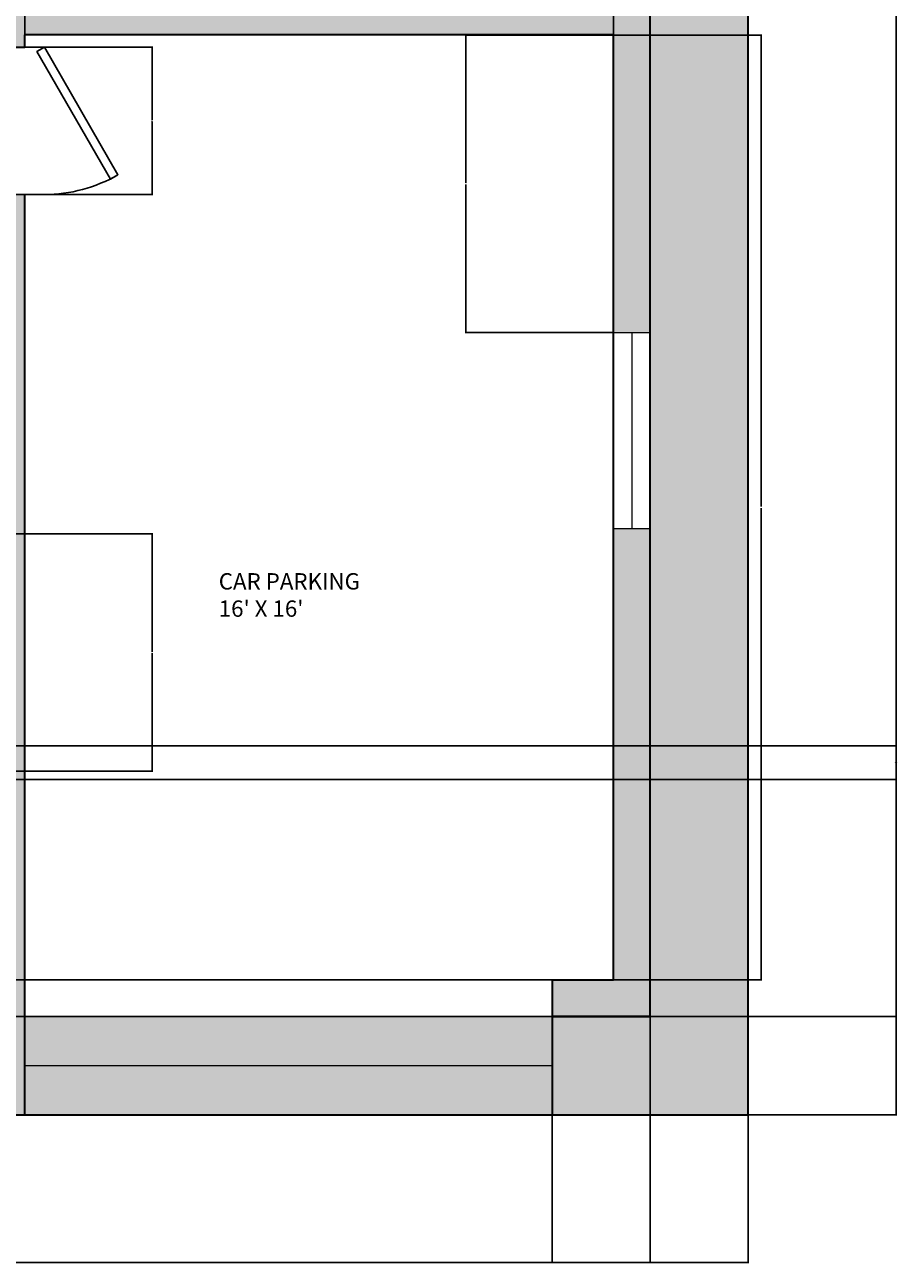
# Model space of a CAD drawing. Units: inches. Extents: x -7 to 546, y -27 to 766.
# Tile 4 of 9: x 332 to 546, y -27 to 276. Entities that reach past the tile are written whole.
import ezdxf

# ---------------------------------------------------------------- set-up
doc = ezdxf.new("R2010")
doc.units = ezdxf.units.IN
doc.header["$MEASUREMENT"] = 0
for name, color, linetype, lineweight in [('A-ANNO-DIMS', 2, 'Continuous', 18), ('A-AREA-IDEN', 7, 'Continuous', 18), ('A-WALL', 7, 'Continuous', 35), ('C-PROP', 7, 'Continuous', 35), ('doors', 40, 'Continuous', 25), ('L-PAVE', 7, 'Continuous', 18), ('window', 30, 'Continuous', 20)]:
    doc.layers.add(name, color=color, linetype=linetype, lineweight=lineweight)
for name, color, linetype, lineweight, true_color in [('A-FLOR-PATT', 143, 'Continuous', 13, 0x7aafdf), ('A-WALL-PATT', 251, 'Continuous', 13, 0x636466), ('L-PLNT-PATT', 85, 'Continuous', 13, 0x58ba48)]:
    doc.layers.add(name, color=color, linetype=linetype, lineweight=lineweight, true_color=true_color)
doc.styles.get("Standard").update_dxf_attribs({"font": 'arial.ttf'})
doc.dimstyles.get("Standard").update_dxf_attribs({"dimtxt": 0.18, "dimasz": 0.18, "dimexe": 0.18, "dimexo": 0.0625, "dimgap": 0.09, "dimtad": 0, "dimtih": 1, "dimtoh": 1, "dimdec": 4, "dimzin": 0, "dimdsep": 46, "dimtxsty": 'Standard', "dimcen": 0.09, "dimadec": 0, "dimazin": 0, "dimtfac": 1, "dimtdec": 4, "dimtofl": 0, "dimtmove": 0, "dimatfit": 3, "dimfxl": 1, "dimtolj": 1, "dimtzin": 0, "dimarcsym": 0})

# ---------------------------------------------------------------- blocks, each defined once
blk = doc.blocks.new('*U10')
for p, q in [((0, 0), (0, -100)), ((750, 0), (750, -100))]:
    blk.add_line(p, q)
blk.add_lwpolyline([(0, 0), (649.5, 375), (671.4, 337.1), (21.9, -37.9)], close=True)
blk.add_arc((0, 0), 750, 0, 30)
blk = doc.blocks.new('WIN-48IN')
for p, q in [((0, 9), (0, 0)), ((48, 9), (0, 9)), ((0, 9), (0, 4.5)), ((48, 0), (48, 9)), ((0, 4.5), (48, 4.5)), ((0, 0), (48, 0))]:
    blk.add_line(p, q)
blk = doc.blocks.new('*D30')
at = {"layer": 'A-ANNO-DIMS', "color": 0, "lineweight": -2, "transparency": 16777216}
for p, q in [((29.23, 9.68), (29.23, -26.56)), ((509.23, 9.68), (509.23, -26.56)), ((29.41, -26.38), (268.94, -26.38)), ((509.05, -26.38), (269.52, -26.38))]:
    blk.add_line(p, q, dxfattribs=at)
at = {"layer": 'A-ANNO-DIMS', "color": 0, "transparency": 16777216}
for points in [[(29.41, -26.35), (29.41, -26.41), (29.23, -26.38)], [(509.05, -26.35), (509.05, -26.41), (509.23, -26.38)]]:
    blk.add_solid(points, dxfattribs=at)
at = {"layer": 'Defpoints', "color": 0, "transparency": 16777216}
for p in [(29.23, 9.74), (509.23, 9.74), (509.23, -26.38)]:
    blk.add_point(p, dxfattribs=at)
at = {"layer": 'A-ANNO-DIMS', "color": 0, "transparency": 16777216, "insert": (269.23, -26.38), "char_height": 0.18, "attachment_point": 5}
blk.add_mtext('\\A1;480', dxfattribs=at)
blk = doc.blocks.new('*D33')
at = {"layer": 'A-ANNO-DIMS', "color": 0, "lineweight": -2, "transparency": 16777216}
for p, q in [((485.29, 705.74), (545.54, 705.74)), ((545.36, 705.56), (545.36, 357.93)), ((545.36, 9.92), (545.36, 357.56)), ((461.29, 9.74), (545.54, 9.74))]:
    blk.add_line(p, q, dxfattribs=at)
at = {"layer": 'A-ANNO-DIMS', "color": 0, "transparency": 16777216}
for points in [[(545.33, 705.56), (545.39, 705.56), (545.36, 705.74)], [(545.33, 9.92), (545.39, 9.92), (545.36, 9.74)]]:
    blk.add_solid(points, dxfattribs=at)
at = {"layer": 'Defpoints', "color": 0, "transparency": 16777216}
for p in [(485.23, 705.74), (461.23, 9.74), (545.36, 9.74)]:
    blk.add_point(p, dxfattribs=at)
at = {"layer": 'A-ANNO-DIMS', "color": 0, "transparency": 16777216, "insert": (545.36, 357.74), "char_height": 0.18, "attachment_point": 5}
blk.add_mtext('\\A1;696', dxfattribs=at)
blk = doc.blocks.new('*D57')
at = {"layer": 'A-ANNO-DIMS', "color": 0, "lineweight": -2, "transparency": 16777216}
for p, q in [((332.23, 273.81), (332.23, 766.05)), ((332.41, 765.87), (403.95, 765.87)), ((476.05, 765.87), (404.51, 765.87)), ((476.23, 273.81), (476.23, 766.05))]:
    blk.add_line(p, q, dxfattribs=at)
at = {"layer": 'A-ANNO-DIMS', "color": 0, "transparency": 16777216}
for points in [[(332.41, 765.9), (332.41, 765.84), (332.23, 765.87)], [(476.05, 765.9), (476.05, 765.84), (476.23, 765.87)]]:
    blk.add_solid(points, dxfattribs=at)
at = {"layer": 'Defpoints', "color": 0, "transparency": 16777216}
for p in [(476.23, 765.87), (332.23, 273.74), (476.23, 273.74)]:
    blk.add_point(p, dxfattribs=at)
at = {"layer": 'A-ANNO-DIMS', "color": 0, "transparency": 16777216, "insert": (404.23, 765.87), "char_height": 0.18, "attachment_point": 5}
blk.add_mtext('\\A1;144', dxfattribs=at)
blk = doc.blocks.new('*D58')
at = {"layer": 'A-ANNO-DIMS', "color": 0, "lineweight": -2, "transparency": 16777216}
for p, q in [((476.29, 273.74), (512.54, 273.74)), ((512.36, 273.56), (512.36, 158.43)), ((512.36, 42.92), (512.36, 158.06)), ((476.29, 42.74), (512.54, 42.74))]:
    blk.add_line(p, q, dxfattribs=at)
at = {"layer": 'A-ANNO-DIMS', "color": 0, "transparency": 16777216}
for points in [[(512.33, 273.56), (512.39, 273.56), (512.36, 273.74)], [(512.33, 42.92), (512.39, 42.92), (512.36, 42.74)]]:
    blk.add_solid(points, dxfattribs=at)
at = {"layer": 'Defpoints', "color": 0, "transparency": 16777216}
for p in [(476.23, 273.74), (476.23, 42.74), (512.36, 42.74)]:
    blk.add_point(p, dxfattribs=at)
at = {"layer": 'A-ANNO-DIMS', "color": 0, "transparency": 16777216, "insert": (512.36, 158.24), "char_height": 0.18, "attachment_point": 5}
blk.add_mtext('\\A1;231', dxfattribs=at)
blk = doc.blocks.new('*D59')
at = {"layer": 'A-ANNO-DIMS', "color": 0, "lineweight": -2, "transparency": 16777216}
for p, q in [((327.29, 151.74), (363.54, 151.74)), ((363.36, 151.56), (363.36, 122.93)), ((363.36, 93.92), (363.36, 122.56)), ((327.29, 93.74), (363.54, 93.74))]:
    blk.add_line(p, q, dxfattribs=at)
at = {"layer": 'A-ANNO-DIMS', "color": 0, "transparency": 16777216}
for points in [[(363.33, 151.56), (363.39, 151.56), (363.36, 151.74)], [(363.33, 93.92), (363.39, 93.92), (363.36, 93.74)]]:
    blk.add_solid(points, dxfattribs=at)
at = {"layer": 'Defpoints', "color": 0, "transparency": 16777216}
for p in [(327.23, 151.74), (327.23, 93.74), (363.36, 93.74)]:
    blk.add_point(p, dxfattribs=at)
at = {"layer": 'A-ANNO-DIMS', "color": 0, "transparency": 16777216, "insert": (363.36, 122.74), "char_height": 0.18, "attachment_point": 5}
blk.add_mtext('\\A1;58', dxfattribs=at)
blk = doc.blocks.new('*D60')
at = {"layer": 'A-ANNO-DIMS', "color": 0, "lineweight": -2, "transparency": 16777216}
for p, q in [((327.29, 270.74), (363.54, 270.74)), ((363.36, 270.56), (363.36, 252.93)), ((363.36, 234.92), (363.36, 252.56)), ((327.29, 234.74), (363.54, 234.74))]:
    blk.add_line(p, q, dxfattribs=at)
at = {"layer": 'A-ANNO-DIMS', "color": 0, "transparency": 16777216}
for points in [[(363.33, 270.56), (363.39, 270.56), (363.36, 270.74)], [(363.33, 234.92), (363.39, 234.92), (363.36, 234.74)]]:
    blk.add_solid(points, dxfattribs=at)
at = {"layer": 'Defpoints', "color": 0, "transparency": 16777216}
for p in [(327.23, 270.74), (327.23, 234.74), (363.36, 234.74)]:
    blk.add_point(p, dxfattribs=at)
at = {"layer": 'A-ANNO-DIMS', "color": 0, "transparency": 16777216, "insert": (363.36, 252.74), "char_height": 0.18, "attachment_point": 5}
blk.add_mtext('\\A1;36', dxfattribs=at)
blk = doc.blocks.new('*D63')
at = {"layer": 'A-ANNO-DIMS', "color": 0, "lineweight": -2, "transparency": 16777216}
for p, q in [((476.17, 273.74), (439.93, 273.74)), ((440.11, 273.56), (440.11, 237.57)), ((440.11, 201.21), (440.11, 237.21)), ((476.17, 201.03), (439.93, 201.03))]:
    blk.add_line(p, q, dxfattribs=at)
at = {"layer": 'A-ANNO-DIMS', "color": 0, "transparency": 16777216}
for points in [[(440.08, 273.56), (440.14, 273.56), (440.11, 273.74)], [(440.08, 201.21), (440.14, 201.21), (440.11, 201.03)]]:
    blk.add_solid(points, dxfattribs=at)
at = {"layer": 'Defpoints', "color": 0, "transparency": 16777216}
for p in [(440.11, 273.74), (476.23, 273.74), (476.23, 201.03)]:
    blk.add_point(p, dxfattribs=at)
at = {"layer": 'A-ANNO-DIMS', "color": 0, "transparency": 16777216, "insert": (440.11, 237.39), "char_height": 0.18, "attachment_point": 5}
blk.add_mtext('\\A1;72.71', dxfattribs=at)
blk = doc.blocks.new('*D64')
at = {"layer": 'A-ANNO-DIMS', "color": 0, "lineweight": -2, "transparency": 16777216}
for p, q in [((461.23, 33.68), (461.23, -26.56)), ((485.23, 33.68), (485.23, -26.56)), ((461.41, -26.38), (473.01, -26.38)), ((485.05, -26.38), (473.45, -26.38))]:
    blk.add_line(p, q, dxfattribs=at)
at = {"layer": 'A-ANNO-DIMS', "color": 0, "transparency": 16777216}
for points in [[(461.41, -26.35), (461.41, -26.41), (461.23, -26.38)], [(485.05, -26.35), (485.05, -26.41), (485.23, -26.38)]]:
    blk.add_solid(points, dxfattribs=at)
at = {"layer": 'Defpoints', "color": 0, "transparency": 16777216}
for p in [(461.23, 33.74), (485.23, 33.74), (461.23, -26.38)]:
    blk.add_point(p, dxfattribs=at)
at = {"layer": 'A-ANNO-DIMS', "color": 0, "transparency": 16777216, "insert": (473.23, -26.38), "char_height": 0.18, "attachment_point": 5}
blk.add_mtext('\\A1;24', dxfattribs=at)
blk = doc.blocks.new('*D65')
at = {"layer": 'A-ANNO-DIMS', "color": 0, "lineweight": -2, "transparency": 16777216}
for p, q in [((461.17, 42.74), (-7.07, 42.74)), ((-6.89, 42.56), (-6.89, 38.43)), ((-6.89, 33.92), (-6.89, 38.06)), ((461.17, 33.74), (-7.07, 33.74))]:
    blk.add_line(p, q, dxfattribs=at)
at = {"layer": 'A-ANNO-DIMS', "color": 0, "transparency": 16777216}
for points in [[(-6.92, 42.56), (-6.86, 42.56), (-6.89, 42.74)], [(-6.92, 33.92), (-6.86, 33.92), (-6.89, 33.74)]]:
    blk.add_solid(points, dxfattribs=at)
at = {"layer": 'Defpoints', "color": 0, "transparency": 16777216}
for p in [(-6.89, 42.74), (461.23, 42.74), (461.23, 33.74)]:
    blk.add_point(p, dxfattribs=at)
at = {"layer": 'A-ANNO-DIMS', "color": 0, "transparency": 16777216, "insert": (-6.89, 38.24), "char_height": 0.18, "attachment_point": 5}
blk.add_mtext('\\A1;9', dxfattribs=at)
blk = doc.blocks.new('*D82')
at = {"layer": 'A-ANNO-DIMS', "color": 0, "lineweight": -2, "transparency": 16777216}
for p, q in [((461.29, 33.74), (545.54, 33.74)), ((545.36, 33.56), (545.36, 21.92)), ((545.36, 9.92), (545.36, 21.56)), ((461.29, 9.74), (545.54, 9.74))]:
    blk.add_line(p, q, dxfattribs=at)
at = {"layer": 'A-ANNO-DIMS', "color": 0, "transparency": 16777216}
for points in [[(545.33, 33.56), (545.39, 33.56), (545.36, 33.74)], [(545.33, 9.92), (545.39, 9.92), (545.36, 9.74)]]:
    blk.add_solid(points, dxfattribs=at)
at = {"layer": 'Defpoints', "color": 0, "transparency": 16777216}
for p in [(461.23, 33.74), (545.36, 33.74), (461.23, 9.74)]:
    blk.add_point(p, dxfattribs=at)
at = {"layer": 'A-ANNO-DIMS', "color": 0, "transparency": 16777216, "insert": (545.36, 21.74), "char_height": 0.18, "attachment_point": 5}
blk.add_mtext('\\A1;24', dxfattribs=at)
blk = doc.blocks.new('*D84')
at = {"layer": 'A-ANNO-DIMS', "color": 0, "lineweight": -2, "transparency": 16777216}
for p, q in [((229.99, 99.94), (545.54, 99.94)), ((545.36, 99.76), (545.36, 96.03)), ((545.36, 91.92), (545.36, 95.66)), ((247.29, 91.74), (545.54, 91.74))]:
    blk.add_line(p, q, dxfattribs=at)
at = {"layer": 'A-ANNO-DIMS', "color": 0, "transparency": 16777216}
for points in [[(545.33, 99.76), (545.39, 99.76), (545.36, 99.94)], [(545.33, 91.92), (545.39, 91.92), (545.36, 91.74)]]:
    blk.add_solid(points, dxfattribs=at)
at = {"layer": 'Defpoints', "color": 0, "transparency": 16777216}
for p in [(229.93, 99.94), (545.36, 99.94), (247.23, 91.74)]:
    blk.add_point(p, dxfattribs=at)
at = {"layer": 'A-ANNO-DIMS', "color": 0, "transparency": 16777216, "insert": (545.36, 95.84), "char_height": 0.18, "attachment_point": 5}
blk.add_mtext('\\A1;8.199', dxfattribs=at)

msp = doc.modelspace()

# ---------------------------------------------------------------- hatches: boundary and pattern name
at = {"layer": 'A-FLOR-PATT'}
h = msp.add_hatch(color=256, dxfattribs=at)
h.dxf.hatch_style = 1
h.paths.add_polyline_path([(252.2319, 33.744), (247.2319, 33.744), (247.2319, 9.744), (332.2319, 9.744), (332.2319, 33.744), (327.2319, 33.744), (327.2319, 13.744), (252.2319, 13.744)])
h = msp.add_hatch(color=256, dxfattribs=at)
h.dxf.hatch_style = 1
h.paths.add_polyline_path([(461.2319, 33.744), (332.2319, 33.744), (332.2319, 21.744), (461.2319, 21.744)])
h.paths.add_polyline_path([(461.2319, 21.744), (332.2319, 21.744), (332.2319, 9.744), (461.2319, 9.744)])
at = {"layer": 'A-WALL-PATT'}
h = msp.add_hatch(color=256, dxfattribs=at)
h.dxf.hatch_style = 1
h.paths.add_polyline_path([(62.2319, 696.744), (86.6896, 696.744), (86.6896, 705.744), (53.2319, 705.744), (53.2319, 627.8642), (57.7271, 627.8642), (62.2319, 627.8642)])
h.paths.add_polyline_path([(229.7414, 705.744), (134.6896, 705.744), (134.6896, 696.744), (206.2319, 696.744), (206.2319, 567.744), (211.2319, 567.744), (211.2319, 595.744), (214.2319, 595.744), (214.2319, 600.744), (211.2319, 600.744), (211.2319, 696.744), (229.7414, 696.744)])
h.paths.add_polyline_path([(293.8423, 705.744), (253.7414, 705.744), (253.7414, 696.744), (274.2319, 696.744), (274.2319, 600.744), (279.2319, 600.744), (279.2319, 696.744), (293.8423, 696.744)])
h.paths.add_polyline_path([(393.9743, 705.744), (317.8423, 705.744), (317.8423, 696.744), (327.2319, 696.744), (327.2319, 651.744), (332.2319, 651.744), (332.2319, 696.744), (393.9743, 696.744)])
h.paths.add_polyline_path([(485.2319, 705.744), (441.9743, 705.744), (441.9743, 696.744), (476.2319, 696.744), (476.2319, 663.6898), (480.7319, 663.6898), (485.2319, 663.6898)])
h.paths.add_polyline_path([(485.2319, 615.6898), (476.2319, 615.6898), (476.2319, 528.744), (332.2319, 528.744), (332.2319, 531.744), (327.2319, 531.744), (327.2319, 523.744), (375.2319, 523.744), (375.2319, 427.744), (327.2319, 427.744), (327.2319, 419.744), (332.2319, 419.744), (332.2319, 422.744), (413.089, 422.744), (413.089, 427.744), (380.2319, 427.744), (380.2319, 523.744), (476.2319, 523.744), (476.2319, 490.9334), (485.2319, 490.9334)])
h.paths.add_polyline_path([(485.2319, 466.9334), (476.2319, 466.9334), (476.2319, 370.0932), (480.7319, 370.0932), (485.2319, 370.0932)])
h.paths.add_polyline_path([(485.2319, 322.0932), (476.2319, 322.0932), (476.2319, 278.744), (332.2319, 278.744), (332.2319, 383.744), (327.2319, 383.744), (327.2319, 273.744), (327.2319, 270.744), (332.2319, 270.744), (332.2319, 273.744), (476.2319, 273.744), (476.2319, 201.0338), (480.7319, 201.0338), (485.2319, 201.0338)])
h.paths.add_polyline_path([(485.2319, 153.0338), (476.2319, 153.0338), (476.2319, 42.744), (461.2319, 42.744), (461.2319, 33.744), (485.2319, 33.744)])
h.paths.add_polyline_path([(332.2319, 234.744), (327.2319, 234.744), (327.2319, 160.744), (315.2319, 160.744), (315.2319, 151.744), (327.2319, 151.744), (327.2319, 33.744), (332.2319, 33.744)])
h.paths.add_polyline_path([(252.2319, 151.744), (258.4464, 151.744), (264.2319, 151.744), (264.2319, 160.744), (252.2319, 160.744), (252.2319, 172.744), (247.2319, 172.744), (247.2319, 91.744), (127.2319, 91.744), (127.2319, 196.744), (122.2319, 196.744), (122.2319, 91.744), (62.2319, 91.744), (62.2319, 126.1124), (53.2319, 126.1124), (53.2319, 9.744), (62.2319, 9.744), (62.2319, 86.744), (247.2319, 86.744), (247.2319, 33.744), (252.2319, 33.744), (252.2319, 53.744)])
h.paths.add_polyline_path([(62.2319, 235.744), (122.2319, 235.744), (122.2319, 232.744), (127.2319, 232.744), (127.2319, 235.744), (247.2319, 235.744), (247.2319, 220.744), (252.2319, 220.744), (252.2319, 240.744), (250.6678, 240.744), (247.2319, 240.744), (62.2319, 240.744), (62.2319, 322.0932), (53.2319, 322.0932), (53.2319, 174.1124), (57.7271, 174.1124), (62.2319, 174.1124)])
at = {"layer": 'L-PLNT-PATT'}
h = msp.add_hatch(color=256, dxfattribs=at)
h.dxf.hatch_style = 1
h.paths.add_polyline_path([(509.2319, 729.744), (29.2319, 729.744), (29.2319, 9.744), (53.2319, 9.744), (53.2319, 705.744), (485.2319, 705.744), (485.2319, 33.744), (461.2319, 33.744), (461.2319, 9.744), (509.2319, 9.744)])

# ---------------------------------------------------------------- linework, layer by layer
at = {"layer": 'A-WALL'}
for p, q in [((332.2319, 270.744), (332.2319, 273.744)), ((476.2319, 273.744), (332.2319, 273.744)), ((476.2319, 42.744), (476.2319, 273.744)), ((327.2319, 270.744), (332.2319, 270.744)), ((332.2319, 9.744), (332.2319, 234.744)), ((461.2319, 42.744), (476.2319, 42.744)), ((461.2319, 42.744), (461.2319, 9.744)), ((485.2319, 33.744), (461.2319, 33.744))]:
    msp.add_line(p, q, dxfattribs=at)
msp.add_lwpolyline([(461.2319, 33.744), (485.2319, 33.744), (485.2319, 705.744), (53.2319, 705.744), (53.2319, 9.744)], dxfattribs=at)
at = {"layer": 'C-PROP'}
msp.add_lwpolyline([(29.2319, 9.744), (509.2319, 9.744), (509.2319, 729.744), (29.2319, 729.744)], close=True, dxfattribs=at)
at = {"layer": 'L-PAVE'}
for p, q in [((332.2319, 33.744), (332.2319, 23.744)), ((332.2319, 33.744), (332.2319, 21.744)), ((332.2319, 21.744), (461.2319, 21.744))]:
    msp.add_line(p, q, dxfattribs=at)
for points in [[(247.2319, 33.744), (332.2319, 33.744)], [(332.2319, 33.744), (461.2319, 33.744)]]:
    msp.add_lwpolyline(points, dxfattribs=at)

# ---------------------------------------------------------------- block references
at = {"layer": 'doors', "xscale": 0.0480000000000013, "yscale": 0.0480000000000013, "zscale": 0.0480000000000013, "rotation": 269.9999999999971}
msp.add_blockref('*U10', (337.0319, 270.744), dxfattribs=at)
at = {"layer": 'window', "extrusion": (0, 0, -1), "zscale": -1, "rotation": 270.0000000000001}
msp.add_blockref('WIN-48IN', (-485.2319, 201.0334), dxfattribs=at)

# ---------------------------------------------------------------- texts
at = {"layer": 'A-AREA-IDEN', "insert": (379.689, 142.1613), "char_height": 4, "attachment_point": 1}
msp.add_mtext_dynamic_manual_height_columns("CAR PARKING\\P16' X 16'", width=80.777321, gutter_width=1, heights=[0], dxfattribs=at)

# ---------------------------------------------------------------- dimensions: what is measured, and where the dimension line sits
at = {"layer": 'A-ANNO-DIMS'}
for base, p1, p2, picture, middle in [((476.2319, 765.869), (332.2319, 273.744), (476.2319, 273.744), '*D57', (404.2319, 765.869)), ((461.2319, -26.381), (485.2319, 33.744), (461.2319, 33.744), '*D64', (473.2319, -26.381)), ((509.2319, -26.381), (29.2319, 9.744), (509.2319, 9.744), '*D30', (269.2319, -26.381))]:
    dim = msp.add_linear_dim(base=base, p1=p1, p2=p2, dimstyle='Standard', override={"dimdec": 0, "dimlfac": 1, "dimrnd": 0, "dimzin": 0, "dimdsep": 46, "dimlunit": 2}, dxfattribs=at)
    dim.commit()
    dim.dimension.update_dxf_attribs({"geometry": picture, "text_midpoint": middle})
for base, p1, p2, angle, override, picture, middle in [((545.3569, 9.744), (485.2319, 705.744), (461.2319, 9.744), 90, {"dimdec": 0, "dimlfac": 1, "dimrnd": 0, "dimzin": 0, "dimdsep": 46, "dimlunit": 2}, '*D33', (545.3569, 357.744)), ((440.1069, 273.744), (476.2319, 201.0338), (476.2319, 273.744), 90, {"dimdec": 2, "dimlfac": 1, "dimrnd": 0, "dimzin": 0, "dimdsep": 46, "dimlunit": 2}, '*D63', (440.1069, 237.3889)), ((512.3569, 42.744), (476.2319, 273.744), (476.2319, 42.744), 270, {"dimdec": 0, "dimlfac": 1, "dimrnd": 0, "dimzin": 0, "dimdsep": 46, "dimlunit": 2}, '*D58', (512.3569, 158.244)), ((363.3569, 234.744), (327.2319, 270.744), (327.2319, 234.744), 270, {"dimdec": 0, "dimlfac": 1, "dimrnd": 0, "dimzin": 0, "dimdsep": 46, "dimlunit": 2}, '*D60', (363.3569, 252.744)), ((363.3569, 93.744), (327.2319, 151.744), (327.2319, 93.744), 270, {"dimdec": 0, "dimlfac": 1, "dimrnd": 0, "dimzin": 0, "dimdsep": 46, "dimlunit": 2}, '*D59', (363.3569, 122.744)), ((545.3569, 99.9426), (247.2319, 91.744), (229.9271, 99.9426), 90, {"dimdec": 3, "dimlfac": 1, "dimrnd": 0, "dimzin": 0, "dimdsep": 46, "dimlunit": 2}, '*D84', (545.3569, 95.8433)), ((-6.8931, 42.744), (461.2319, 33.744), (461.2319, 42.744), 90, {"dimdec": 0, "dimlfac": 1, "dimrnd": 0, "dimzin": 0, "dimdsep": 46, "dimlunit": 2}, '*D65', (-6.8931, 38.244)), ((545.3569, 33.744), (461.2319, 9.744), (461.2319, 33.744), 90, {"dimdec": 0, "dimlfac": 1, "dimrnd": 0, "dimzin": 0, "dimdsep": 46, "dimlunit": 2}, '*D82', (545.3569, 21.744))]:
    dim = msp.add_linear_dim(base=base, p1=p1, p2=p2, angle=angle, dimstyle='Standard', override=override, dxfattribs=at)
    dim.commit()
    dim.dimension.update_dxf_attribs({"geometry": picture, "text_midpoint": middle})

doc.saveas('drawing.dxf')
